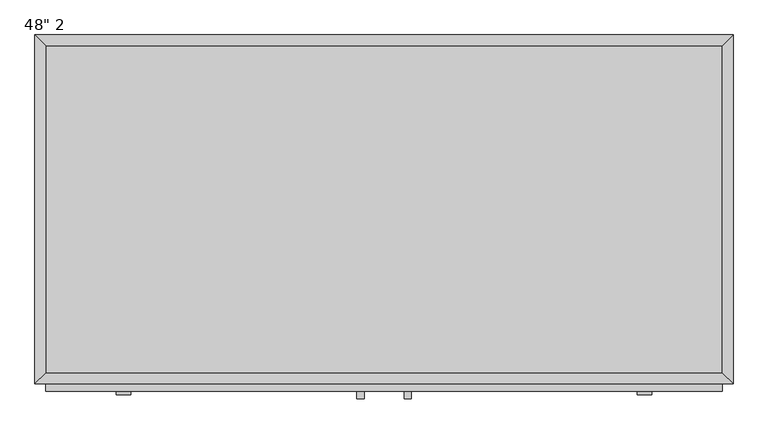
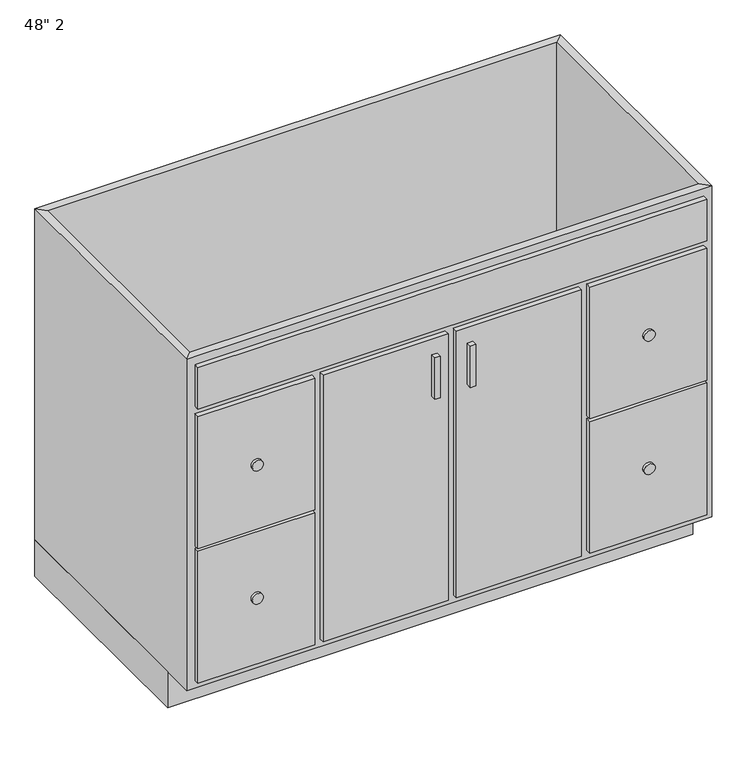
"""IFC4 building model written with IfcOpenShell, lengths in millimetres: furniture geometry."""

from ifc_helpers import new_model, si_unit, point, frame, frame_2d, origin, origin_with_axes, place, context, project, spatial, polyline, circle_curve, trimmed, segment, composite_curve, outline, extrude, faceted_brep, source, transform, mapped, element, save


def furniture_b04c6994(model_context):
    return source(origin(), model_context, "Body", "SolidModel", [
        extrude(outline(polyline([(700.44496, 0.0), (700.44496, -533.4), (-518.75504, -533.4), (-518.75504, 0.0), (700.44496, 0.0)])), origin_with_axes(), (0.0, 0.0, 1.0), 88.9),
        faceted_brep([(681.39496, -590.55, 901.7), (681.39496, -590.55, 88.9), (-499.70504, -590.55, 88.9), (-499.70504, -590.55, 901.7), (700.44496, -609.6, 901.7), (-518.75504, -609.6, 901.7), (700.44496, -609.6, 88.9), (-518.75504, -609.6, 88.9), (-499.70504, -19.05, 88.9), (-499.70504, -19.05, 901.7), (-518.75504, 0.0, 901.7), (-518.75504, 0.0, 88.9), (681.39496, -19.05, 88.9), (681.39496, -19.05, 901.7), (700.44496, 0.0, 901.7), (700.44496, 0.0, 88.9)], [[[0, 1, 2, 3]], [[4, 0, 3, 5]], [[6, 4, 5, 7]], [[1, 6, 7, 2]], [[3, 2, 8, 9]], [[5, 3, 9, 10]], [[7, 5, 10, 11]], [[2, 7, 11, 8]], [[9, 8, 12, 13]], [[10, 9, 13, 14]], [[11, 10, 14, 15]], [[8, 11, 15, 12]], [[13, 12, 1, 0]], [[14, 13, 0, 4]], [[15, 14, 4, 6]], [[12, 15, 6, 1]]]),
        extrude(outline(polyline([(681.39496, -19.05), (681.39496, -590.55), (-499.70504, -590.55), (-499.70504, -19.05), (681.39496, -19.05)])), frame((0.0, 0.0, 88.9), z_axis=(0.0, 0.0, 1.0), x_axis=(1.0, 0.0, 0.0)), (0.0, 0.0, 1.0), 19.05),
        extrude(outline(composite_curve([segment(trimmed(circle_curve(frame_2d((271.4625, 545.66371)), 12.7), [point((271.4625, 532.96371))], [point((271.4625, 558.36371))], False, "CARTESIAN"), True, "CONTINUOUS"), segment(trimmed(circle_curve(frame_2d((271.4625, 545.66371)), 12.7), [point((271.4625, 558.36371))], [point((271.4625, 532.96371))], False, "CARTESIAN"), True, "CONTINUOUS")], self_intersect=False)), frame((0.0, -628.65, 0.0), z_axis=(0.0, 1.0, 0.0), x_axis=(0.0, 0.0, 1.0)), (0.0, 0.0, 1.0), 6.35),
        extrude(outline(composite_curve([segment(trimmed(circle_curve(frame_2d((598.4875, 545.66371)), 12.7), [point((598.4875, 532.96371))], [point((598.4875, 558.36371))], False, "CARTESIAN"), True, "CONTINUOUS"), segment(trimmed(circle_curve(frame_2d((598.4875, 545.66371)), 12.7), [point((598.4875, 558.36371))], [point((598.4875, 532.96371))], False, "CARTESIAN"), True, "CONTINUOUS")], self_intersect=False)), frame((0.0, -628.65, 0.0), z_axis=(0.0, 1.0, 0.0), x_axis=(0.0, 0.0, 1.0)), (0.0, 0.0, 1.0), 6.35),
        extrude(outline(composite_curve([segment(trimmed(circle_curve(frame_2d((598.4875, -363.97379)), 12.7), [point((598.4875, -376.67379))], [point((598.4875, -351.27379))], False, "CARTESIAN"), True, "CONTINUOUS"), segment(trimmed(circle_curve(frame_2d((598.4875, -363.97379)), 12.7), [point((598.4875, -351.27379))], [point((598.4875, -376.67379))], False, "CARTESIAN"), True, "CONTINUOUS")], self_intersect=False)), frame((0.0, -628.65, 0.0), z_axis=(0.0, 1.0, 0.0), x_axis=(0.0, 0.0, 1.0)), (0.0, 0.0, 1.0), 6.35),
        extrude(outline(composite_curve([segment(trimmed(circle_curve(frame_2d((271.4625, -363.97379)), 12.7), [point((271.4625, -376.67379))], [point((271.4625, -351.27379))], False, "CARTESIAN"), True, "CONTINUOUS"), segment(trimmed(circle_curve(frame_2d((271.4625, -363.97379)), 12.7), [point((271.4625, -351.27379))], [point((271.4625, -376.67379))], False, "CARTESIAN"), True, "CONTINUOUS")], self_intersect=False)), frame((0.0, -628.65, 0.0), z_axis=(0.0, 1.0, 0.0), x_axis=(0.0, 0.0, 1.0)), (0.0, 0.0, 1.0), 6.35),
        extrude(outline(polyline([(55.91996, -635.0), (43.21996, -635.0), (43.21996, -622.3), (55.91996, -622.3), (55.91996, -635.0)])), frame((0.0, 0.0, 622.3), z_axis=(0.0, 0.0, 1.0), x_axis=(1.0, 0.0, 0.0)), (0.0, 0.0, 1.0), 101.6),
        extrude(outline(polyline([(138.46996, -635.0), (125.76996, -635.0), (125.76996, -622.3), (138.46996, -622.3), (138.46996, -635.0)])), frame((0.0, 0.0, 622.3), z_axis=(0.0, 0.0, 1.0), x_axis=(1.0, 0.0, 0.0)), (0.0, 0.0, 1.0), 101.6),
        extrude(outline(polyline([(681.39496, -622.3), (-499.70504, -622.3), (-499.70504, -609.6), (681.39496, -609.6), (681.39496, -622.3)])), frame((0.0, 0.0, 781.05), z_axis=(0.0, 0.0, 1.0), x_axis=(1.0, 0.0, 0.0)), (0.0, 0.0, 1.0), 101.6),
        extrude(outline(polyline([(681.39496, -622.3), (409.93246, -622.3), (409.93246, -609.6), (681.39496, -609.6), (681.39496, -622.3)])), frame((0.0, 0.0, 438.15), z_axis=(0.0, 0.0, 1.0), x_axis=(1.0, 0.0, 0.0)), (0.0, 0.0, 1.0), 323.85),
        extrude(outline(polyline([(681.39496, -622.3), (409.93246, -622.3), (409.93246, -609.6), (681.39496, -609.6), (681.39496, -622.3)])), frame((0.0, 0.0, 107.95), z_axis=(0.0, 0.0, 1.0), x_axis=(1.0, 0.0, 0.0)), (0.0, 0.0, 1.0), 323.85),
        extrude(outline(polyline([(-228.24254, -622.3), (-499.70504, -622.3), (-499.70504, -609.6), (-228.24254, -609.6), (-228.24254, -622.3)])), frame((0.0, 0.0, 438.15), z_axis=(0.0, 0.0, 1.0), x_axis=(1.0, 0.0, 0.0)), (0.0, 0.0, 1.0), 323.85),
        extrude(outline(polyline([(-228.24254, -622.3), (-499.70504, -622.3), (-499.70504, -609.6), (-228.24254, -609.6), (-228.24254, -622.3)])), frame((0.0, 0.0, 107.95), z_axis=(0.0, 0.0, 1.0), x_axis=(1.0, 0.0, 0.0)), (0.0, 0.0, 1.0), 323.85),
        extrude(outline(polyline([(81.31996, -622.3), (-209.19254, -622.3), (-209.19254, -609.6), (81.31996, -609.6), (81.31996, -622.3)])), frame((0.0, 0.0, 107.95), z_axis=(0.0, 0.0, 1.0), x_axis=(1.0, 0.0, 0.0)), (0.0, 0.0, 1.0), 654.05),
        extrude(outline(polyline([(390.88246, -622.3), (100.36996, -622.3), (100.36996, -609.6), (390.88246, -609.6), (390.88246, -622.3)])), frame((0.0, 0.0, 107.95), z_axis=(0.0, 0.0, 1.0), x_axis=(1.0, 0.0, 0.0)), (0.0, 0.0, 1.0), 654.05),
    ])


if __name__ == "__main__":
    model = new_model("IFC4")
    model_context = context("Model", 3, world=origin())
    ifc_project = project(units=[si_unit("LENGTHUNIT", "METRE", prefix="MILLI")], contexts=[model_context])
    site = spatial("IfcSite", under=ifc_project)
    building = spatial("IfcBuilding", under=site)
    placement = place(None, origin())
    furniture_shape = furniture_b04c6994(model_context)
    element("IfcFurniture", 1, ObjectType="48\" 2", at=placement, inside=building, context=model_context, shape_type="MappedRepresentation", body=[
        mapped(furniture_shape, transform((0.0, 0.0, 0.0), x_axis=(1.0, 0.0, 0.0), y_axis=(0.0, 1.0, 0.0), z_axis=(0.0, 0.0, 1.0))),
    ])
    save(model, "model.ifc")

# Revit data of these elements
# Type "48\" 2"
#   Assembly Code = "C1030410"
#   Depth = 2' - 0"
#   Height = 2' - 11 1/2"
#   Toe Depth = 0' - 3"
#   Toe Height = 0' - 3 1/2"
#   Width = 4' - 0"
#   Cabinet Material = none
#   Door/Drawer Material = none
#   Handle Material = Cabinets - Handles
#   Default Elevation = 0
# Element 1 (IfcFurniture, "48\" 2")
#   Materials on its faces: "Cabinets", "Cabinets - Handles"
# Materials
#   "Cabinets - Handles": colour RGB 57 57 57, transparency 0
#   "Cabinets": colour RGB 249 249 249, transparency 0
